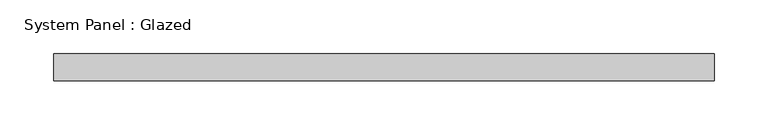
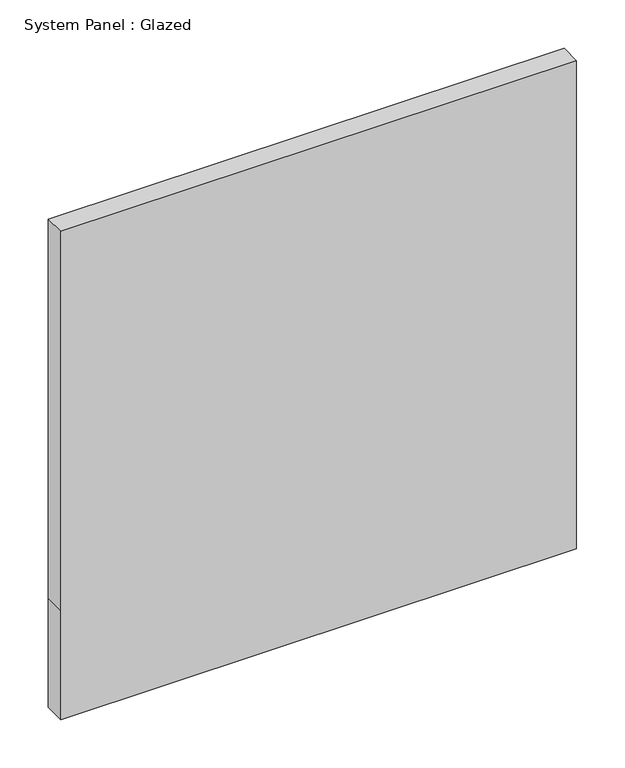
"""IFC4 building model written with IfcOpenShell, lengths in millimetres: plate geometry, System Panel : Glazed."""

from ifc_helpers import new_model, si_unit, frame, origin, place, context, project, spatial, polyline, outline, extrude, source, transform, mapped, element, save


def system_panel_glazed_776d8ebc(model_context):
    return source(origin(), model_context, "Body", "SweptSolid", [
        extrude(outline(polyline([(0.0, -307.975), (0.0, 307.975), (137.7374164, 307.975), (616.4122491, 307.975), (616.4122491, -307.975), (137.7374164, -307.975), (0.0, -307.975)])), frame((0.0, 19.05, 0.0), z_axis=(0.0, 1.0, 0.0), x_axis=(0.0, 0.0, 1.0)), (0.0, 0.0, 1.0), 25.4),
    ])


if __name__ == "__main__":
    model = new_model("IFC4")
    model_context = context("Model", 3, world=origin())
    ifc_project = project(units=[si_unit("LENGTHUNIT", "METRE", prefix="MILLI")], contexts=[model_context])
    site = spatial("IfcSite", under=ifc_project)
    building = spatial("IfcBuilding", under=site)
    placement = place(None, origin())
    system_panel_glazed_shape = system_panel_glazed_776d8ebc(model_context)
    element("IfcPlate", 1, ObjectType="System Panel : Glazed", at=placement, inside=building, context=model_context, shape_type="MappedRepresentation", body=[
        mapped(system_panel_glazed_shape, transform((0.0, 0.0, 0.0), x_axis=(1.0, 0.0, 0.0), y_axis=(0.0, 1.0, 0.0), z_axis=(0.0, 0.0, 1.0))),
    ])
    save(model, "model.ifc")

# Revit data of these elements
# Type "System Panel : Glazed"
#   Construction Type Id = "GSP4R"
#   Analytic Construction = "1/8 in Pilkington single glazing"
#   Visual Light Transmittance = 0.9
#   Solar Heat Gain Coefficient = 0.86
#   Heat Transfer Coefficient (U) = 1.18115 BTU/(h·ft²·°F)
#   Define Thermal Properties by = 1
# Element 1 (IfcPlate, "System Panel : Glazed")
#   Materials on its faces: "Glass"
# Materials
#   "Glass": class "Glass", colour RGB 0 128 192, transparency 0.75, Description = "Soda Lime Glass", Cost = 0
